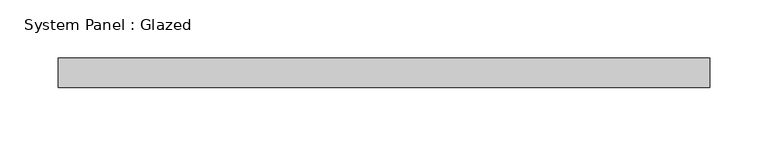
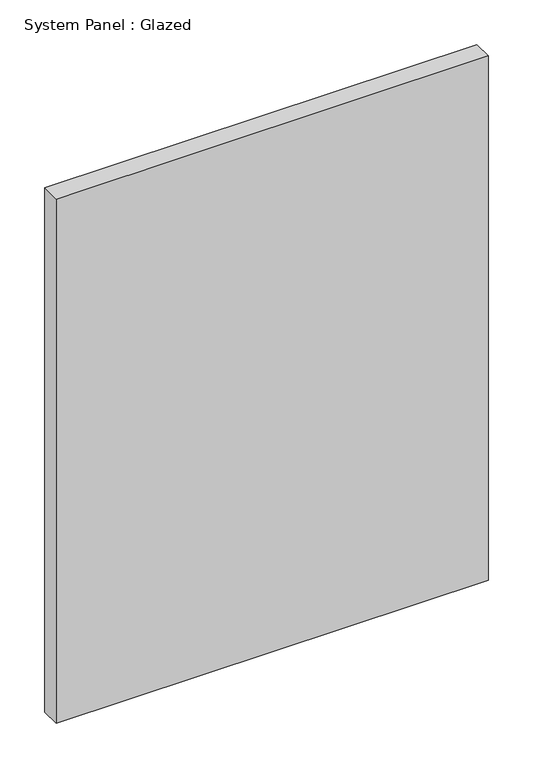
"""IFC4 building model written with IfcOpenShell, lengths in millimetres: plate geometry, System Panel : Glazed."""

from ifc_helpers import new_model, si_unit, origin, origin_with_axes, place, context, project, spatial, polyline, outline, extrude, source, transform, mapped, element, save


def system_panel_glazed_ffb4b76a(model_context):
    return source(origin(), model_context, "Body", "SweptSolid", [
        extrude(outline(polyline([(279.4, 19.05), (-279.4, 19.05), (-279.4, 44.45), (279.4, 44.45), (279.4, 19.05)])), origin_with_axes(), (0.0, 0.0, 1.0), 716.4323007),
    ])


if __name__ == "__main__":
    model = new_model("IFC4")
    model_context = context("Model", 3, world=origin())
    ifc_project = project(units=[si_unit("LENGTHUNIT", "METRE", prefix="MILLI")], contexts=[model_context])
    site = spatial("IfcSite", under=ifc_project)
    building = spatial("IfcBuilding", under=site)
    placement = place(None, origin())
    system_panel_glazed_shape = system_panel_glazed_ffb4b76a(model_context)
    element("IfcPlate", 1, ObjectType="System Panel : Glazed", at=placement, inside=building, context=model_context, shape_type="MappedRepresentation", body=[
        mapped(system_panel_glazed_shape, transform((0.0, 0.0, 0.0), x_axis=(1.0, 0.0, 0.0), y_axis=(0.0, 1.0, 0.0), z_axis=(0.0, 0.0, 1.0))),
    ])
    save(model, "model.ifc")

# Revit data of these elements
# Type "System Panel : Glazed"
#   Construction Type Id = "GSP4R"
#   Analytic Construction = "1/8 in Pilkington single glazing"
#   Visual Light Transmittance = 0.9
#   Solar Heat Gain Coefficient = 0.86
#   Heat Transfer Coefficient (U) = 1.18115 BTU/(h·ft²·°F)
#   Define Thermal Properties by = 1
# Element 1 (IfcPlate, "System Panel : Glazed")
#   Materials on its faces: "Glass"
# Materials
#   "Glass": class "Glass", colour RGB 0 128 192, transparency 0.75, Description = "Soda Lime Glass", Cost = 0
